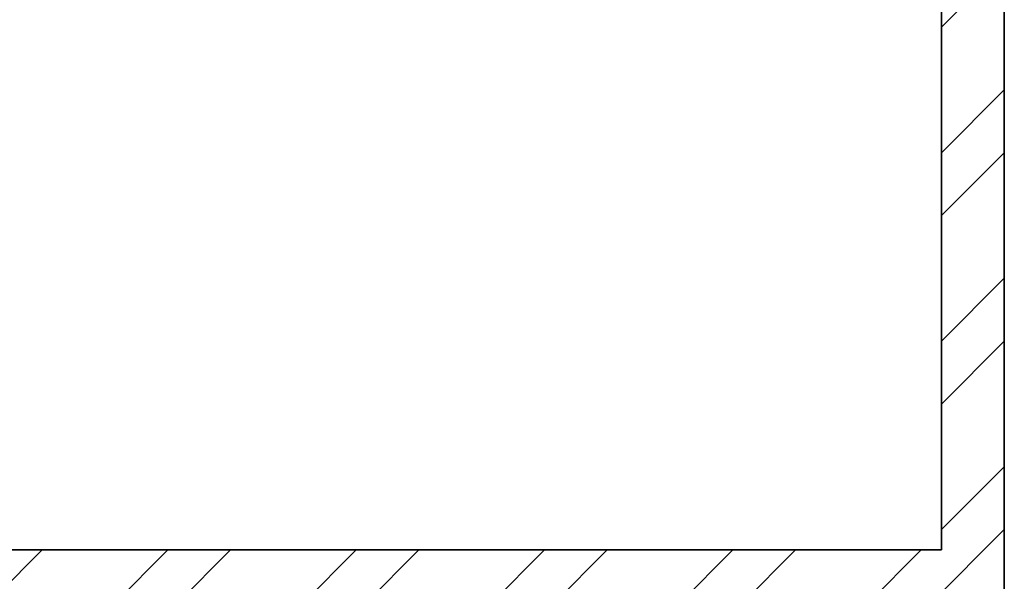
# Model space of a CAD drawing. Units: inches. Extents: x 1962 to 2771, y 1245 to 2660.
# Tile 72 of 114: x 2590 to 2661, y 1979 to 2019. Entities that reach past the tile are written whole.
import ezdxf

# ---------------------------------------------------------------- set-up
doc = ezdxf.new("R2010")
doc.units = ezdxf.units.IN
doc.layers.add('A-WALL', color=7, linetype='Continuous', lineweight=35)
doc.layers.add('A-WALL-PATT', color=252, linetype='Continuous', lineweight=13)

msp = doc.modelspace()

# ---------------------------------------------------------------- hatches: boundary and pattern name
at = {"layer": 'A-WALL-PATT'}
h = msp.add_hatch(dxfattribs=at)
h.set_pattern_fill('ANSI32', color=256)
h.paths.add_polyline_path([(2090.8074, 2467.3437), (2141.6481, 2467.3437), (2141.6481, 2469.5937), (2141.6481, 2471.8437), (2086.3074, 2471.8437), (2086.3074, 2422.5333), (2090.8074, 2422.5333)])
h.paths.add_polyline_path([(2282.7664, 2471.8437), (2204.8982, 2471.8437), (2204.8982, 2467.3437), (2234.8074, 2467.3437), (2234.8074, 2311.3437), (2228.7492, 2311.3437), (2228.7492, 2306.8437), (2234.8074, 2306.8437), (2331.9227, 2306.8437), (2331.9227, 2309.0937), (2331.9227, 2311.3437), (2239.3074, 2311.3437), (2239.3074, 2467.3437), (2282.7664, 2467.3437), (2282.7664, 2469.5937)])
h.paths.add_polyline_path([(2471.4531, 2519.8437), (2552.011, 2519.8437), (2564.3996, 2519.8437), (2564.3996, 2511.1389), (2568.8996, 2511.1389), (2568.8996, 2524.3437), (2466.9531, 2524.3437), (2466.9531, 2471.8437), (2450.0749, 2471.8437), (2446.4672, 2471.8437), (2446.4672, 2467.3437), (2450.0749, 2467.3437), (2475.9988, 2467.3437), (2475.9988, 2469.5937), (2475.9988, 2471.8437), (2471.4531, 2471.8437)])
h.paths.add_polyline_path([(2575.2231, 2469.5937), (2575.2231, 2471.8437), (2568.8996, 2471.8437), (2568.8996, 2487.1389), (2564.3996, 2487.1389), (2564.3996, 2471.8437), (2556.511, 2471.8437), (2499.2904, 2471.8437), (2499.2904, 2467.3437), (2507.8074, 2467.3437), (2507.8074, 2311.3437), (2414.863, 2311.3437), (2414.863, 2306.8437), (2512.3074, 2306.8437), (2517.0114, 2306.8437), (2517.0114, 2309.0937), (2517.0114, 2311.3437), (2512.3074, 2311.3437), (2512.3074, 2467.3437), (2575.2231, 2467.3437)])
h.paths.add_polyline_path([(2660.8074, 2471.8437), (2600.9602, 2471.8437), (2600.9602, 2467.3437), (2656.3074, 2467.3437), (2656.3074, 2432.5704), (2660.8074, 2432.5704)])
h.paths.add_polyline_path([(2660.8074, 2372.5704), (2656.3074, 2372.5704), (2656.3074, 2311.3437), (2600.276, 2311.3437), (2600.276, 2309.0937), (2600.276, 2306.8437), (2656.3074, 2306.8437), (2656.3074, 2296.2593), (2660.8074, 2296.2593)])
h.paths.add_polyline_path([(2572.3074, 2306.8437), (2577.1385, 2306.8437), (2577.1385, 2311.3437), (2551.082, 2311.3437), (2551.082, 2306.8437), (2567.8074, 2306.8437), (2567.8074, 2258.8437), (2540.0574, 2258.8437), (2540.0574, 2256.5937), (2540.0574, 2254.3437), (2567.8074, 2254.3437), (2656.3074, 2254.3437), (2656.3074, 2236.9085), (2660.8074, 2236.9085), (2660.8074, 2272.2593), (2656.3074, 2272.2593), (2656.3074, 2258.8437), (2572.3074, 2258.8437)])
h.paths.add_polyline_path([(2512.3074, 2254.3437), (2518.8716, 2254.3437), (2518.8716, 2256.5937), (2518.8716, 2258.8437), (2507.8074, 2258.8437), (2507.8074, 2177.8437), (2567.8074, 2177.8437), (2567.8074, 2172.9628), (2572.3074, 2172.9628), (2572.3074, 2177.8437), (2656.3074, 2177.8437), (2656.3074, 2166.4846), (2660.8074, 2166.4846), (2660.8074, 2200.9085), (2656.3074, 2200.9085), (2656.3074, 2182.3437), (2512.3074, 2182.3437)])
h.paths.add_polyline_path([(2656.3074, 2129.8437), (2572.3074, 2129.8437), (2572.3074, 2150.3044), (2570.0574, 2150.3044), (2567.8074, 2150.3044), (2567.8074, 2129.8437), (2507.8074, 2129.8437), (2507.8074, 2116.3027), (2510.0574, 2116.3027), (2512.3074, 2116.3027), (2512.3074, 2125.3437), (2567.8074, 2125.3437), (2572.3074, 2125.3437), (2656.3074, 2125.3437)])
h.paths.add_polyline_path([(2090.8074, 2362.5333), (2086.3074, 2362.5333), (2086.3074, 2298.6242), (2090.8074, 2298.6242), (2090.8074, 2306.8437), (2174.8074, 2306.8437), (2174.8074, 2286.4178), (2179.3074, 2286.4178), (2179.3074, 2306.8437), (2192.8641, 2306.8437), (2192.8641, 2309.0937), (2192.8641, 2311.3437), (2090.8074, 2311.3437)])
h.paths.add_polyline_path([(2209.156, 2258.8437), (2179.3074, 2258.8437), (2179.3074, 2263.2236), (2177.0574, 2263.2236), (2174.8074, 2263.2236), (2174.8074, 2258.8437), (2090.8074, 2258.8437), (2090.8074, 2274.6242), (2086.3074, 2274.6242), (2086.3074, 2238.2967), (2088.5574, 2238.2967), (2090.8074, 2238.2967), (2090.8074, 2254.3437), (2209.156, 2254.3437)])
h.paths.add_polyline_path([(2090.8074, 2177.8437), (2234.8074, 2177.8437), (2234.8074, 2173.1428), (2239.3074, 2173.1428), (2239.3074, 2258.8437), (2230.8442, 2258.8437), (2230.8442, 2256.5937), (2230.8442, 2254.3437), (2234.8074, 2254.3437), (2234.8074, 2182.3437), (2090.8074, 2182.3437), (2090.8074, 2202.2967), (2086.3074, 2202.2967), (2086.3074, 2140.0389), (2090.8074, 2140.0389)])
h.paths.add_polyline_path([(2090.8074, 2080.0389), (2086.3074, 2080.0389), (2086.3074, 2033.8437), (2090.8074, 2033.8437)], flags=17)
h.paths.add_polyline_path([(2244.9405, 2033.8437), (2239.3074, 2033.8437), (2239.3074, 2142.0665), (2237.2592, 2142.0665), (2234.8074, 2142.0665), (2234.8074, 2033.8437), (2090.8074, 2033.8437), (2076.5204, 2033.8437), (2072.0204, 2033.8437), (2072.0204, 2000.4493), (2076.5204, 2000.4493), (2076.5204, 2029.3437), (2090.8074, 2029.3437), (2244.9405, 2029.3437), (2244.9405, 2031.5937)])
h.paths.add_polyline_path([(2234.8074, 1933.3437), (2076.5204, 1933.3437), (2076.5204, 1952.4493), (2074.2704, 1952.4493), (2072.0204, 1952.4493), (2072.0204, 1933.3437), (2072.0204, 1928.8437), (2234.8074, 1928.8437)])
h.paths.add_polyline_path([(2090.8074, 1928.8437), (2086.3074, 1928.8437), (2086.3074, 1906.5013), (2090.8074, 1906.5013)])
h.paths.add_polyline_path([(2090.8074, 1846.5013), (2086.3074, 1846.5013), (2086.3074, 1769.9917), (2088.5574, 1769.9917), (2090.8074, 1769.9917), (2090.8074, 1780.3437), (2234.8074, 1780.3437), (2234.8074, 1708.3437), (2230.3764, 1708.3437), (2230.3764, 1703.8437), (2239.3074, 1703.8437), (2239.3074, 1792.6669), (2237.0574, 1792.6669), (2234.8074, 1792.6669), (2234.8074, 1784.8437), (2090.8074, 1784.8437)])
h.paths.add_polyline_path([(2239.3074, 1928.8437), (2244.9405, 1928.8437), (2244.9405, 1931.0937), (2244.9405, 1933.3437), (2234.8074, 1933.3437), (2234.8074, 1928.8437), (2234.8074, 1825.5949), (2239.3074, 1825.5949)])
h.paths.add_polyline_path([(2148.0425, 1649.0937), (2148.0425, 1651.3437), (2090.8074, 1651.3437), (2090.8074, 1646.8437), (2148.0425, 1646.8437)], flags=0)
h.paths.add_polyline_path([(2207.5601, 1708.3437), (2090.8074, 1708.3437), (2090.8074, 1703.8437), (2174.8074, 1703.8437), (2174.8074, 1651.3437), (2170.4457, 1651.3437), (2170.4457, 1646.8437), (2195.9924, 1646.8437), (2195.9924, 1649.0937), (2195.9924, 1651.3437), (2179.3074, 1651.3437), (2179.3074, 1703.8437), (2207.5601, 1703.8437), (2207.5601, 1706.0937)])
h.paths.add_polyline_path([(2090.8074, 1733.9917), (2086.3074, 1733.9917), (2086.3074, 1696.1032), (2088.5574, 1696.1032), (2090.8074, 1696.1032)])
h.paths.add_polyline_path([(2090.8074, 1672.1032), (2086.3074, 1672.1032), (2086.3074, 1600.3335), (2090.8074, 1600.3335)])
h.paths.add_polyline_path([(2090.8074, 1540.3335), (2086.3074, 1540.3335), (2086.3074, 1486.3437), (2139.6766, 1486.3437), (2139.6766, 1490.8437), (2090.8074, 1490.8437)])
h.paths.add_polyline_path([(2302.3876, 1490.8437), (2239.3074, 1490.8437), (2239.3074, 1646.8437), (2335.9994, 1646.8437), (2335.9994, 1651.3437), (2229.884, 1651.3437), (2229.884, 1646.8437), (2234.8074, 1646.8437), (2234.8074, 1490.8437), (2202.7103, 1490.8437), (2202.7103, 1488.5937), (2202.7103, 1486.3437), (2275.0699, 1486.3437), (2275.0699, 1475.772), (2279.5699, 1475.772), (2279.5699, 1486.3437), (2302.3876, 1486.3437)])
h.paths.add_polyline_path([(2279.5699, 1451.772), (2275.0699, 1451.772), (2275.0699, 1438.3437), (2174.8074, 1438.3437), (2174.8074, 1486.3437), (2179.7922, 1486.3437), (2179.7922, 1490.8437), (2163.3585, 1490.8437), (2163.3585, 1488.5937), (2163.3585, 1486.3437), (2170.3074, 1486.3437), (2170.3074, 1433.8437), (2279.5699, 1433.8437)])
h.paths.add_polyline_path([(2427.2363, 1490.8437), (2375.8074, 1490.8437), (2375.8074, 1646.8437), (2381.6401, 1646.8437), (2381.6401, 1651.3437), (2365.887, 1651.3437), (2365.887, 1649.0937), (2365.887, 1646.8437), (2371.3074, 1646.8437), (2371.3074, 1490.8437), (2327.5627, 1490.8437), (2327.5627, 1488.5937), (2327.5627, 1486.3437), (2371.3074, 1486.3437), (2371.3074, 1433.8437), (2375.8074, 1433.8437), (2375.8074, 1486.3437), (2427.2363, 1486.3437)])
h.paths.add_polyline_path([(2512.3074, 1646.8437), (2519.4351, 1646.8437), (2519.4351, 1649.0937), (2519.4351, 1651.3437), (2507.8074, 1651.3437), (2416.0063, 1651.3437), (2416.0063, 1649.0937), (2416.0063, 1646.8437), (2507.8074, 1646.8437), (2507.8074, 1490.8437), (2497.0532, 1490.8437), (2497.0532, 1488.5937), (2497.0532, 1486.3437), (2574.9344, 1486.3437), (2574.9344, 1476.0181), (2579.4344, 1476.0181), (2579.4344, 1486.3437), (2584.4872, 1486.3437), (2584.3074, 1490.8437), (2512.3074, 1490.8437)])
h.paths.add_polyline_path([(2470.5091, 1486.3437), (2473.9767, 1486.3437), (2473.9767, 1490.8437), (2449.6605, 1490.8437), (2449.6605, 1488.5937), (2449.6605, 1486.3437), (2466.0091, 1486.3437), (2466.0091, 1433.8437), (2470.5091, 1433.8437), (2579.4344, 1433.8437), (2579.4344, 1452.0181), (2574.9344, 1452.0181), (2574.9344, 1438.3437), (2554.5091, 1438.3437), (2470.5091, 1438.3437)])
h.paths.add_polyline_path([(2656.3074, 1490.8437), (2611.86, 1490.8437), (2611.86, 1486.3437), (2656.3074, 1486.3437)])
h.paths.add_polyline_path([(2660.8074, 1532.7007), (2658.5574, 1532.7007), (2656.3074, 1532.7007), (2656.3074, 1486.3437), (2660.8074, 1486.3437)])
h.paths.add_polyline_path([(2660.8074, 1664.9663), (2656.3074, 1664.9663), (2656.3074, 1651.3437), (2602.2313, 1651.3437), (2602.2313, 1646.8437), (2656.3074, 1646.8437), (2656.3074, 1592.7007), (2660.8074, 1592.7007)])
h.paths.add_polyline_path([(2660.8074, 1724.5221), (2656.3074, 1724.5221), (2656.3074, 1703.8437), (2542.4725, 1703.8437), (2542.4725, 1699.3437), (2567.8074, 1699.3437), (2567.8074, 1651.3437), (2552.7766, 1651.3437), (2552.7766, 1649.0937), (2552.7766, 1646.8437), (2577.2878, 1646.8437), (2577.2878, 1649.0937), (2577.2878, 1651.3437), (2572.3074, 1651.3437), (2572.3074, 1699.3437), (2656.3074, 1699.3437), (2656.3074, 1688.9663), (2660.8074, 1688.9663)])
h.paths.add_polyline_path([(2660.8074, 1880.6524), (2656.3074, 1880.6524), (2656.3074, 1832.8437), (2512.3074, 1832.8437), (2512.3074, 1837.8959), (2507.8074, 1837.8959), (2507.8074, 1828.3437), (2567.8074, 1828.3437), (2567.8074, 1804.3437), (2572.3074, 1804.3437), (2572.3074, 1828.3437), (2656.3074, 1828.3437), (2656.3074, 1818.6778), (2660.8074, 1818.6778)])
h.paths.add_polyline_path([(2660.8074, 1794.6778), (2656.3074, 1794.6778), (2656.3074, 1780.3437), (2572.3074, 1780.3437), (2572.3074, 1783.0303), (2570.0574, 1783.0303), (2567.8074, 1783.0303), (2567.8074, 1780.3437), (2507.8074, 1780.3437), (2507.8074, 1699.3437), (2517.8858, 1699.3437), (2517.8858, 1701.5937), (2517.8858, 1703.8437), (2512.3074, 1703.8437), (2512.3074, 1775.8437), (2656.3074, 1775.8437), (2656.3074, 1760.5221), (2660.8074, 1760.5221)])
h.paths.add_polyline_path([(2660.8074, 1981.3437), (2660.8074, 2020.2808), (2658.5574, 2020.2808), (2656.3074, 2020.2808), (2656.3074, 1981.3437), (2512.3074, 1981.3437), (2512.3074, 2086.6996), (2507.8074, 2086.6996), (2507.8074, 1981.3437), (2375.8074, 1981.3437), (2375.8074, 1986.8505), (2373.5574, 1986.8505), (2371.3074, 1986.8505), (2371.3074, 1973.2607), (2375.8074, 1973.2607), (2375.8074, 1976.8437), (2507.8074, 1976.8437), (2507.8074, 1865.4281), (2510.0574, 1865.4281), (2512.3074, 1865.4281), (2512.3074, 1976.8437), (2660.8074, 1976.8437)])
h.paths.add_polyline_path([(2375.8074, 1940.297), (2373.5574, 1940.297), (2371.3074, 1940.297), (2371.3074, 1933.3437), (2278.4434, 1933.3437), (2278.4434, 1928.8437), (2371.3074, 1928.8437), (2371.3074, 1651.3437), (2375.8074, 1651.3437)])
h.paths.add_polyline_path([(2660.8074, 1976.8437), (2656.3074, 1976.8437), (2656.3074, 1940.6524), (2660.8074, 1940.6524)], flags=17)
h.paths.add_polyline_path([(2660.8074, 2142.4846), (2656.3074, 2142.4846), (2656.3074, 2080.2808), (2660.8074, 2080.2808)])
h.paths.add_polyline_path([(2381.4189, 2311.3437), (2375.8074, 2311.3437), (2375.8074, 2467.3437), (2424.7242, 2467.3437), (2424.7242, 2469.5937), (2424.7242, 2471.8437), (2375.8074, 2471.8437), (2375.8074, 2524.3437), (2371.3074, 2524.3437), (2371.3074, 2471.8437), (2307.2097, 2471.8437), (2307.2097, 2467.3437), (2371.3074, 2467.3437), (2371.3074, 2311.3437), (2366.8901, 2311.3437), (2366.8901, 2306.8437), (2371.3074, 2306.8437), (2371.3074, 2033.8437), (2279.6589, 2033.8437), (2279.6589, 2029.3437), (2371.3074, 2029.3437), (2371.3074, 2014.2598), (2375.8074, 2014.2598), (2375.8074, 2306.8437), (2381.4189, 2306.8437)])
h.paths.add_polyline_path([(2263.3074, 2524.3437), (2170.3074, 2524.3437), (2170.3074, 2519.8437), (2170.3074, 2471.8437), (2165.0312, 2471.8437), (2165.0312, 2467.3437), (2179.6721, 2467.3437), (2179.6721, 2469.5161), (2179.6721, 2471.8437), (2174.8074, 2471.8437), (2174.8074, 2519.8437), (2258.8074, 2519.8437), (2258.8074, 2511.6436), (2263.3074, 2511.6436)])
h.paths.add_polyline_path([(2245.0232, 1361.4123), (2492.9468, 1361.4123), (2492.9468, 1398.505), (2245.0232, 1398.505)], flags=9)
h.paths.add_polyline_path([(2388.1434, 2086.6936), (2425.0704, 2086.6936), (2425.0704, 2105.3509), (2388.1434, 2105.3509)], flags=9)
h.paths.add_polyline_path([(2404.922, 2242.6744), (2445.7337, 2242.6744), (2445.7337, 2261.3318), (2404.922, 2261.3318)], flags=9)
h.paths.add_polyline_path([(2269.4107, 2156.7935), (2306.3378, 2156.7935), (2306.3378, 2175.4508), (2269.4107, 2175.4508)], flags=9)
h.paths.add_polyline_path([(2269.3277, 2233.4343), (2306.2547, 2233.4343), (2306.2547, 2252.0917), (2269.3277, 2252.0917)], flags=9)
h.paths.add_polyline_path([(2431.6052, 2320.6922), (2470.4456, 2320.6922), (2470.4456, 2339.3495), (2431.6052, 2339.3495)], flags=25)
h.paths.add_polyline_path([(2249.6902, 2315.7608), (2288.5306, 2315.7608), (2288.5306, 2334.4182), (2249.6902, 2334.4182)], flags=25)
h.paths.add_polyline_path([(2096.9301, 2314.3181), (2135.7704, 2314.3181), (2135.7704, 2332.9755), (2096.9301, 2332.9755)], flags=25)
h.paths.add_polyline_path([(2134.3475, 2285.7089), (2161.4655, 2285.7089), (2161.4655, 2304.3662), (2134.3475, 2304.3662)], flags=9)
h.paths.add_polyline_path([(2126.5155, 2209.4076), (2159.9227, 2209.4076), (2159.9227, 2228.065), (2126.5155, 2228.065)], flags=25)
h.paths.add_polyline_path([(2110.5753, 2141.5299), (2149.4157, 2141.5299), (2149.4157, 2160.1872), (2110.5753, 2160.1872)], flags=25)
h.paths.add_polyline_path([(2249.8618, 1968.3317), (2286.3966, 1968.3317), (2286.3966, 1986.989), (2249.8618, 1986.989)], flags=9)
h.paths.add_polyline_path([(2395.9507, 1777.0051), (2436.7624, 1777.0051), (2436.7624, 1795.6625), (2395.9507, 1795.6625)], flags=9)
h.paths.add_polyline_path([(2398.5259, 1888.5651), (2435.0062, 1888.5651), (2435.0062, 1907.2224), (2398.5259, 1907.2224)], flags=25)
h.paths.add_polyline_path([(2259.3506, 1728.3559), (2296.2776, 1728.3559), (2296.2776, 1747.0132), (2259.3506, 1747.0132)], flags=9)
h.paths.add_polyline_path([(2271.3698, 1845.268), (2308.2968, 1845.268), (2308.2968, 1863.9253), (2271.3698, 1863.9253)], flags=9)
h.paths.add_polyline_path([(2120.9355, 1786.3027), (2159.7759, 1786.3027), (2159.7759, 1804.9601), (2120.9355, 1804.9601)], flags=25)
h.paths.add_polyline_path([(2121.3164, 1732.1043), (2154.7236, 1732.1043), (2154.7236, 1750.7616), (2121.3164, 1750.7616)], flags=25)
h.paths.add_polyline_path([(2118.3706, 1678.8997), (2147.5282, 1678.8997), (2147.5282, 1697.557), (2118.3706, 1697.557)], flags=25)
h.paths.add_polyline_path([(2385.9227, 1493.557), (2424.763, 1493.557), (2424.763, 1512.2143), (2385.9227, 1512.2143)], flags=25)
h.paths.add_polyline_path([(2248.7058, 1500.0256), (2287.5462, 1500.0256), (2287.5462, 1518.6829), (2248.7058, 1518.6829)], flags=25)
h.paths.add_polyline_path([(2104.1669, 1617.3771), (2143.0073, 1617.3771), (2143.0073, 1636.0344), (2104.1669, 1636.0344)], flags=9)
h.paths.add_polyline_path([(2096.0714, 1447.8824), (2137.3845, 1447.8824), (2137.3845, 1458.1859), (2096.0714, 1458.1859)], flags=9)
h.paths.add_polyline_path([(2180.6114, 1440.325), (2209.7689, 1440.325), (2209.7689, 1458.9823), (2180.6114, 1458.9823)], flags=25)
h.paths.add_polyline_path([(2316.1698, 1447.9637), (2357.4829, 1447.9637), (2357.4829, 1458.2673), (2316.1698, 1458.2673)], flags=9)
h.paths.add_polyline_path([(2397.6187, 1447.9637), (2438.9318, 1447.9637), (2438.9318, 1458.2673), (2397.6187, 1458.2673)], flags=9)
h.paths.add_polyline_path([(2473.0778, 1439.5953), (2502.2354, 1439.5953), (2502.2354, 1458.2527), (2473.0778, 1458.2527)], flags=25)
h.paths.add_polyline_path([(2589.7027, 1447.8819), (2631.0158, 1447.8819), (2631.0158, 1458.1855), (2589.7027, 1458.1855)], flags=9)
h.paths.add_polyline_path([(2522.4009, 1497.5285), (2561.2413, 1497.5285), (2561.2413, 1516.1859), (2522.4009, 1516.1859)], flags=25)
h.paths.add_polyline_path([(2579.6565, 1671.3482), (2608.8141, 1671.3482), (2608.8141, 1690.0056), (2579.6565, 1690.0056)], flags=25)
h.paths.add_polyline_path([(2544.7038, 1725.5064), (2578.1111, 1725.5064), (2578.1111, 1744.1637), (2544.7038, 1744.1637)], flags=25)
h.paths.add_polyline_path([(2578.1191, 1807.472), (2607.2766, 1807.472), (2607.2766, 1826.1293), (2578.1191, 1826.1293)], flags=25)
h.paths.add_polyline_path([(2595.0614, 1835.1839), (2633.9018, 1835.1839), (2633.9018, 1853.8413), (2595.0614, 1853.8413)], flags=25)
h.paths.add_polyline_path([(2567.0097, 2097.7035), (2605.8501, 2097.7035), (2605.8501, 2116.3609), (2567.0097, 2116.3609)], flags=9)
h.paths.add_polyline_path([(2586.644, 2134.6454), (2615.8015, 2134.6454), (2615.8015, 2153.3027), (2586.644, 2153.3027)], flags=9)
h.paths.add_polyline_path([(2544.6185, 2212.6783), (2578.0258, 2212.6783), (2578.0258, 2231.3356), (2544.6185, 2231.3356)], flags=25)
h.paths.add_polyline_path([(2577.0273, 2256.9023), (2606.1849, 2256.9023), (2606.1849, 2275.5597), (2577.0273, 2275.5597)], flags=24)
h.paths.add_polyline_path([(2605.2683, 2315.2821), (2644.1087, 2315.2821), (2644.1087, 2333.9395), (2605.2683, 2333.9395)], flags=25)
h.paths.add_polyline_path([(2583.1244, 2496.1815), (2624.4375, 2496.1815), (2624.4375, 2506.4851), (2583.1244, 2506.4851)], flags=9)
h.paths.add_polyline_path([(2474.761, 2497.0823), (2503.9185, 2497.0823), (2503.9185, 2515.7397), (2474.761, 2515.7397)], flags=25)
h.paths.add_polyline_path([(2387.5787, 2494.2563), (2428.902, 2494.2563), (2428.902, 2504.5598), (2387.5787, 2504.5598)], flags=9)
h.paths.add_polyline_path([(2300.1657, 2500.1564), (2341.4788, 2500.1564), (2341.4788, 2510.46), (2300.1657, 2510.46)], flags=25)
h.paths.add_polyline_path([(2176.8589, 2497.5843), (2206.0165, 2497.5843), (2206.0165, 2516.2416), (2176.8589, 2516.2416)], flags=25)
h.paths.add_polyline_path([(2097.4668, 2494.9762), (2138.7799, 2494.9762), (2138.7799, 2505.2798), (2097.4668, 2505.2798)], flags=9)

# ---------------------------------------------------------------- linework, layer by layer
at = {"layer": 'A-WALL'}
for p, q in [((2660.8074, 2471.8437), (2660.8074, 1976.8437)), ((2656.3074, 2177.8437), (2656.3074, 1981.3437)), ((2512.3074, 1981.3437), (2656.3074, 1981.3437)), ((2660.8074, 1981.3437), (2660.8074, 1976.8437))]:
    msp.add_line(p, q, dxfattribs=at)

doc.saveas('drawing.dxf')
